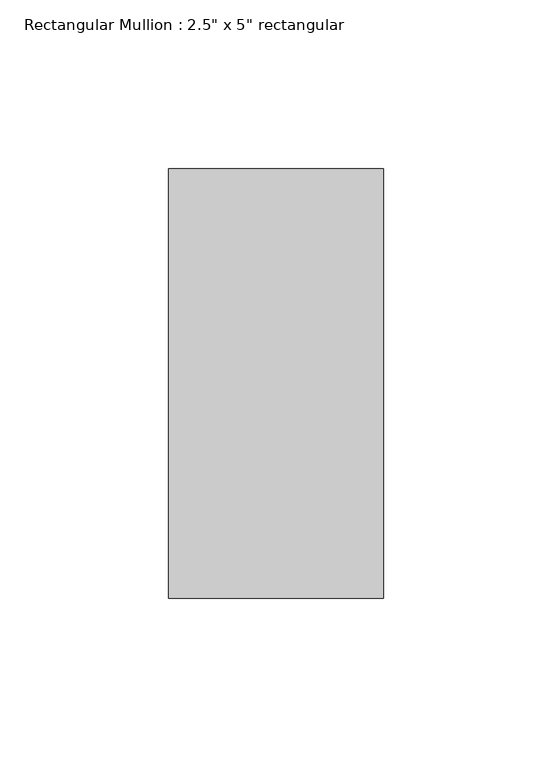
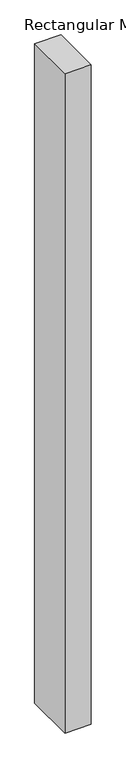
"""IFC4 building model written with IfcOpenShell, lengths in millimetres: member geometry."""

from ifc_helpers import new_model, si_unit, frame, origin, place, context, project, spatial, polyline, outline, extrude, source, transform, mapped, element, save


def member_0a25ecd0(model_context):
    return source(origin(), model_context, "Body", "SweptSolid", [
        extrude(outline(polyline([(31.75, 63.5), (31.75, -63.5), (-31.75, -63.5), (-31.75, 63.5), (31.75, 63.5)])), frame((0.0, 0.0, -1693.6943888), z_axis=(0.0, 0.0, 1.0), x_axis=(1.0, 0.0, 0.0)), (0.0, 0.0, 1.0), 1693.6943888),
    ])


if __name__ == "__main__":
    model = new_model("IFC4")
    model_context = context("Model", 3, world=origin())
    ifc_project = project(units=[si_unit("LENGTHUNIT", "METRE", prefix="MILLI")], contexts=[model_context])
    site = spatial("IfcSite", under=ifc_project)
    building = spatial("IfcBuilding", under=site)
    placement = place(None, origin())
    member_shape = member_0a25ecd0(model_context)
    element("IfcMember", 1, ObjectType="Rectangular Mullion : 2.5\" x 5\" rectangular", at=placement, inside=building, context=model_context, shape_type="MappedRepresentation", body=[
        mapped(member_shape, transform((0.0, 0.0, 0.0), x_axis=(1.0, 0.0, 0.0), y_axis=(0.0, 1.0, 0.0), z_axis=(0.0, 0.0, 1.0))),
    ])
    save(model, "model.ifc")

# Revit data of these elements
# Type "Rectangular Mullion : 2.5\" x 5\" rectangular"
#   built-in parameter 1007304 = 0.416667 (stored number, unit not read)
#   built-in parameter 1007301 = 0.104167 (stored number, unit not read)
#   built-in parameter 1007300 = 0.104167 (stored number, unit not read)
# Element 1 (IfcMember, "Rectangular Mullion : 2.5\" x 5\" rectangular")
#   Materials on its faces: "Aluminum"
# Materials
#   "Aluminum": class "Metal", colour RGB 247 247 247, transparency 0, Description = "Aluminum 6061", Cost = 0
